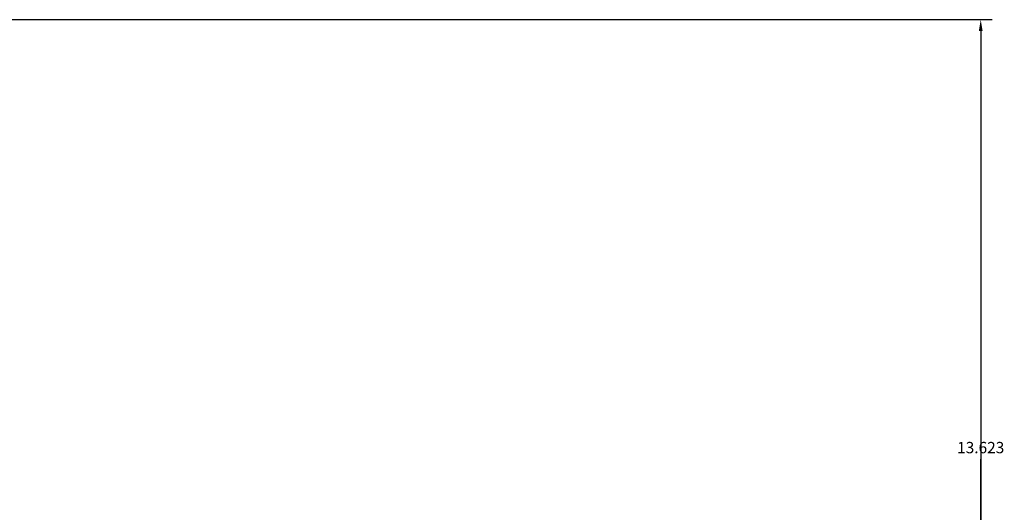
# Model space of a CAD drawing. Units: inches. Extents: x -6 to 289, y -8 to 323.
# Tile 107 of 107: x 273.2 to 288.85, y 299.45 to 307.29. Entities that reach past the tile are written whole.
import ezdxf

# ---------------------------------------------------------------- set-up
doc = ezdxf.new("R2010")
doc.units = ezdxf.units.IN
doc.header["$MEASUREMENT"] = 0
doc.layers.add('A-ANNO-DIMS', color=2, linetype='Continuous', lineweight=18)
doc.styles.get("Standard").update_dxf_attribs({"font": 'arial.ttf'})
doc.dimstyles.get("Standard").update_dxf_attribs({"dimtxt": 0.18, "dimasz": 0.18, "dimexe": 0.18, "dimexo": 0.0625, "dimgap": 0.09, "dimtad": 0, "dimtih": 1, "dimtoh": 1, "dimdec": 4, "dimzin": 0, "dimdsep": 46, "dimtxsty": 'Standard', "dimcen": 0.09, "dimadec": 0, "dimazin": 0, "dimtfac": 1, "dimtdec": 4, "dimtofl": 0, "dimtmove": 0, "dimatfit": 3, "dimfxl": 1, "dimtolj": 1, "dimtzin": 0, "dimarcsym": 0})

# ---------------------------------------------------------------- blocks, each defined once
blk = doc.blocks.new('*D27')
at = {"layer": 'A-ANNO-DIMS', "color": 0, "lineweight": -2, "transparency": 16777216}
for p, q in [((19.226, 307.289), (288.653, 307.289)), ((288.473, 307.109), (288.473, 277.471)), ((288.473, 247.469), (288.473, 277.107)), ((247.226, 247.289), (288.653, 247.289))]:
    blk.add_line(p, q, dxfattribs=at)
at = {"layer": 'A-ANNO-DIMS', "color": 0, "transparency": 16777216}
for points in [[(288.443, 307.109), (288.503, 307.109), (288.473, 307.289)], [(288.443, 247.469), (288.503, 247.469), (288.473, 247.289)]]:
    blk.add_solid(points, dxfattribs=at)
at = {"layer": 'Defpoints', "color": 0, "transparency": 16777216}
for p in [(19.164, 307.289), (288.473, 307.289), (247.164, 247.289)]:
    blk.add_point(p, dxfattribs=at)
at = {"layer": 'A-ANNO-DIMS', "color": 0, "transparency": 16777216, "insert": (288.473, 277.289), "char_height": 0.18, "attachment_point": 5}
blk.add_mtext('\\A1;60', dxfattribs=at)
blk = doc.blocks.new('*D118')
at = {"layer": 'A-ANNO-DIMS', "color": 0, "lineweight": -2, "transparency": 16777216}
for p, q in [((118.226, 307.289), (288.653, 307.289)), ((288.473, 307.109), (288.473, 300.659)), ((288.473, 293.846), (288.473, 300.295)), ((257.703, 293.666), (288.653, 293.666))]:
    blk.add_line(p, q, dxfattribs=at)
at = {"layer": 'A-ANNO-DIMS', "color": 0, "transparency": 16777216}
for points in [[(288.443, 307.109), (288.503, 307.109), (288.473, 307.289)], [(288.443, 293.846), (288.503, 293.846), (288.473, 293.666)]]:
    blk.add_solid(points, dxfattribs=at)
at = {"layer": 'Defpoints', "color": 0, "transparency": 16777216}
for p in [(118.164, 307.289), (288.473, 307.289), (257.641, 293.666)]:
    blk.add_point(p, dxfattribs=at)
at = {"layer": 'A-ANNO-DIMS', "color": 0, "transparency": 16777216, "insert": (288.473, 300.477), "char_height": 0.18, "attachment_point": 5}
blk.add_mtext('\\A1;13.623', dxfattribs=at)

msp = doc.modelspace()

# ---------------------------------------------------------------- dimensions: what is measured, and where the dimension line sits
at = {"layer": 'A-ANNO-DIMS'}
for p1, p2, override, picture, middle in [((247.1638, 247.2888), (19.1638, 307.2888), {"dimdec": 0, "dimlfac": 1, "dimrnd": 0, "dimzin": 0, "dimdsep": 46, "dimlunit": 2}, '*D27', (288.4733, 277.2888)), ((257.6407, 293.6657), (118.1638, 307.2888), {"dimdec": 3, "dimlfac": 1, "dimrnd": 0, "dimzin": 0, "dimdsep": 46, "dimlunit": 2}, '*D118', (288.4733, 300.4773))]:
    dim = msp.add_linear_dim(base=(288.4733, 307.2888), p1=p1, p2=p2, angle=90, dimstyle='Standard', override=override, dxfattribs=at)
    dim.commit()
    dim.dimension.update_dxf_attribs({"geometry": picture, "text_midpoint": middle})

doc.saveas('drawing.dxf')
